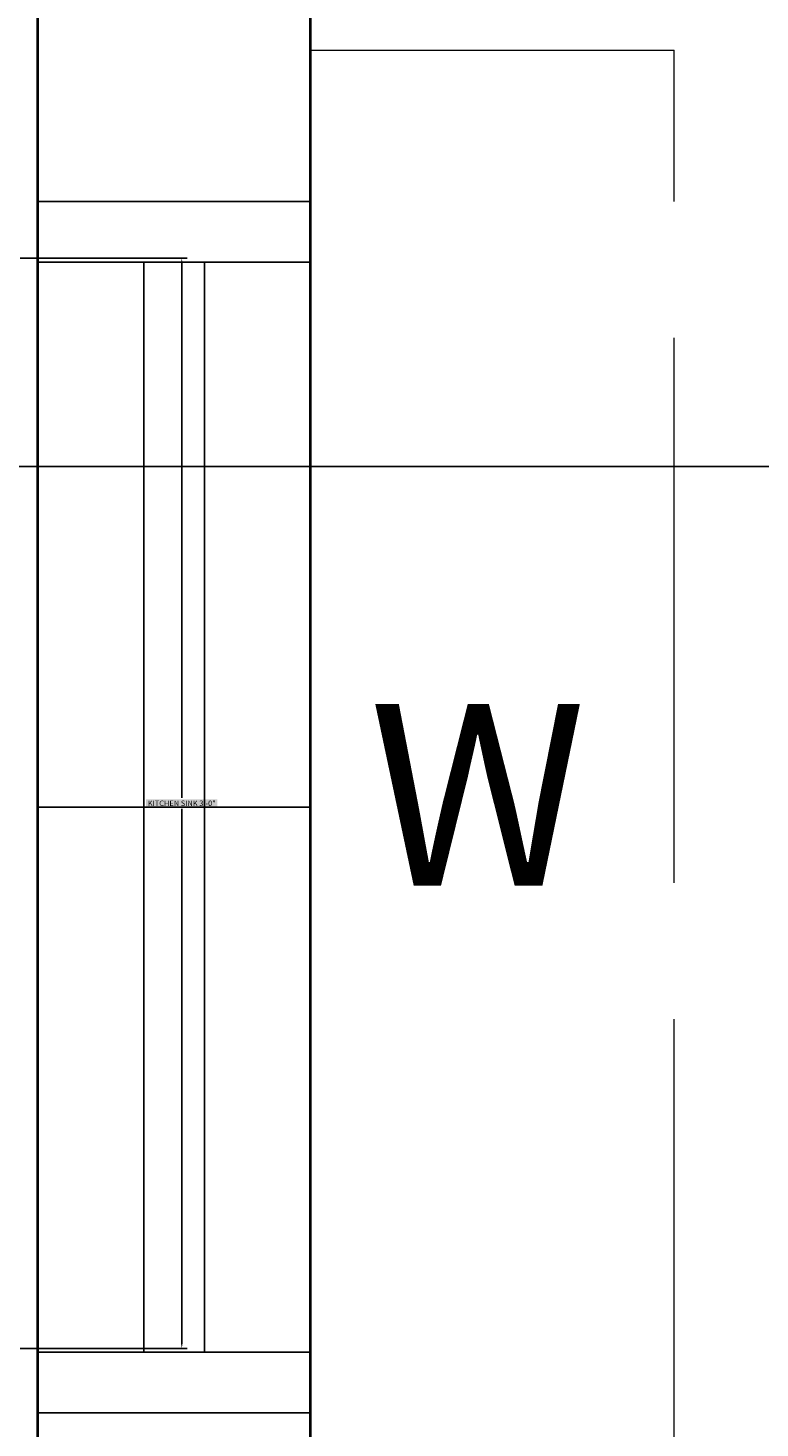
# Model space of a CAD drawing. Units: inches. Extents: x -301 to 715, y -607 to 364.
# Tile 122 of 141: x 124 to 148, y 230 to 276. Entities that reach past the tile are written whole.
import ezdxf

# ---------------------------------------------------------------- set-up
doc = ezdxf.new("R2010")
doc.units = ezdxf.units.IN
doc.header["$MEASUREMENT"] = 0
doc.linetypes.add('ACAD_ISO02W100', pattern=[15, 12, -3])
for name, color, linetype, lineweight in [('A-ANNO-DIMS', 2, 'Continuous', 18), ('A-ANNO-TEXT', 4, 'Continuous', 18), ('A-GLAZ', 2, 'Continuous', 25), ('A-GLAZ-OVHD', 2, 'ACAD_ISO02W100', 18), ('A-WALL', 3, 'Continuous', 40)]:
    doc.layers.add(name, color=color, linetype=linetype, lineweight=lineweight)
doc.styles.get("Standard").update_dxf_attribs({"font": 'arial.ttf'})
doc.dimstyles.get("Standard").update_dxf_attribs({"dimtxt": 0.18, "dimasz": 0.18, "dimexe": 0.18, "dimexo": 0.0625, "dimgap": 0.09, "dimtad": 0, "dimtih": 1, "dimtoh": 1, "dimdec": 1, "dimzin": 0, "dimdsep": 46, "dimlunit": 4, "dimtxsty": 'Standard', "dimcen": 0.09, "dimclrd": 3, "dimclre": 4, "dimclrt": 6, "dimadec": 0, "dimazin": 0, "dimtfac": 1, "dimtdec": 1, "dimtofl": 0, "dimtmove": 0, "dimatfit": 3, "dimfxl": 1, "dimtfill": 2, "dimtfillclr": 51, "dimtolj": 1, "dimtzin": 0, "dimarcsym": 0})

# ---------------------------------------------------------------- blocks, each defined once
blk = doc.blocks.new('WIN-36-PLAN')
for p, q in [((0, 0), (0, 9)), ((2, 0), (2, 9)), ((20, 0), (20, 9)), ((38, 0), (38, 9)), ((40, 0), (40, 9)), ((2, 5.5), (38, 5.5)), ((2, 3.5), (38, 3.5))]:
    blk.add_line(p, q)
blk = doc.blocks.new('WIN-SHADE-50')
at = {"ltscale": 1.5}
for p, q in [((0, 0), (0, 12)), ((50, 12), (0, 12)), ((5, 0), (0, 0)), ((45, 0), (50, 0))]:
    blk.add_line(p, q, dxfattribs=at)
blk = doc.blocks.new('*D142')
at = {"layer": 'A-ANNO-DIMS', "color": 4, "lineweight": -2, "transparency": 16777216}
for p, q in [((123.308, 268.311), (128.826, 268.311)), ((123.308, 232.311), (128.826, 232.311))]:
    blk.add_line(p, q, dxfattribs=at)
at = {"layer": 'A-ANNO-DIMS', "color": 3, "lineweight": -2, "transparency": 16777216}
for p, q in [((128.646, 268.131), (128.646, 250.494)), ((128.646, 232.491), (128.646, 250.128))]:
    blk.add_line(p, q, dxfattribs=at)
at = {"layer": 'A-ANNO-DIMS', "color": 3, "transparency": 16777216}
for points in [[(128.616, 268.131), (128.676, 268.131), (128.646, 268.311)], [(128.616, 232.491), (128.676, 232.491), (128.646, 232.311)]]:
    blk.add_solid(points, dxfattribs=at)
at = {"layer": 'Defpoints', "color": 0, "transparency": 16777216}
for p in [(123.246, 268.311), (128.646, 268.311), (123.246, 232.311)]:
    blk.add_point(p, dxfattribs=at)
at = {"layer": 'A-ANNO-DIMS', "color": 6, "transparency": 16777216, "insert": (128.646, 250.311), "char_height": 0.18, "attachment_point": 5, "bg_fill": 1, "box_fill_scale": 1.25, "bg_fill_color": 51, "bg_fill_transparency": 0}
blk.add_mtext('\\A1;KITCHEN SINK 3\'-0"', dxfattribs=at)
blk = doc.blocks.new('*D153')
at = {"layer": 'A-ANNO-DIMS', "color": 4, "lineweight": -2, "transparency": 16777216}
for p, q in [((132.959, 310.182), (233.659, 310.182)), ((123.959, 193.182), (233.659, 193.182))]:
    blk.add_line(p, q, dxfattribs=at)
at = {"layer": 'A-ANNO-DIMS', "color": 3, "lineweight": -2, "transparency": 16777216}
for p, q in [((233.479, 310.002), (233.479, 251.864)), ((233.479, 193.362), (233.479, 251.5))]:
    blk.add_line(p, q, dxfattribs=at)
at = {"layer": 'A-ANNO-DIMS', "color": 3, "transparency": 16777216}
for points in [[(233.449, 310.002), (233.509, 310.002), (233.479, 310.182)], [(233.449, 193.362), (233.509, 193.362), (233.479, 193.182)]]:
    blk.add_solid(points, dxfattribs=at)
at = {"layer": 'Defpoints', "color": 0, "transparency": 16777216}
for p in [(132.897, 310.182), (123.897, 193.182), (233.479, 193.182)]:
    blk.add_point(p, dxfattribs=at)
at = {"layer": 'A-ANNO-DIMS', "color": 6, "transparency": 16777216, "insert": (233.479, 251.682), "char_height": 0.18, "attachment_point": 5, "bg_fill": 1, "box_fill_scale": 1.25, "bg_fill_color": 51, "bg_fill_transparency": 0}
blk.add_mtext('\\A1;9\'-9"', dxfattribs=at)
blk = doc.blocks.new('*D157')
at = {"layer": 'A-ANNO-DIMS', "color": 4, "lineweight": -2, "transparency": 16777216}
for p, q in [((-50.541, 261.432), (233.659, 261.432)), ((-50.541, 221.682), (233.659, 221.682))]:
    blk.add_line(p, q, dxfattribs=at)
at = {"layer": 'A-ANNO-DIMS', "color": 3, "lineweight": -2, "transparency": 16777216}
for p, q in [((233.479, 261.252), (233.479, 241.739)), ((233.479, 221.862), (233.479, 241.375))]:
    blk.add_line(p, q, dxfattribs=at)
at = {"layer": 'A-ANNO-DIMS', "color": 3, "transparency": 16777216}
for points in [[(233.449, 261.252), (233.509, 261.252), (233.479, 261.432)], [(233.449, 221.862), (233.509, 221.862), (233.479, 221.682)]]:
    blk.add_solid(points, dxfattribs=at)
at = {"layer": 'Defpoints', "color": 0, "transparency": 16777216}
for p in [(-50.603, 261.432), (233.479, 261.432), (-50.603, 221.682)]:
    blk.add_point(p, dxfattribs=at)
at = {"layer": 'A-ANNO-DIMS', "color": 6, "transparency": 16777216, "insert": (233.479, 241.557), "char_height": 0.18, "attachment_point": 5, "bg_fill": 1, "box_fill_scale": 1.25, "bg_fill_color": 51, "bg_fill_transparency": 0}
blk.add_mtext('\\A1;3\'-4"', dxfattribs=at)

msp = doc.modelspace()

# ---------------------------------------------------------------- linework, layer by layer
at = {"layer": 'A-WALL'}
for p, q in [((132.897, 199.182), (132.897, 310.182)), ((123.897, 199.182), (123.897, 301.182))]:
    msp.add_line(p, q, dxfattribs=at)

# ---------------------------------------------------------------- block references
at = {"layer": 'A-GLAZ', "rotation": 90.00000000000026}
msp.add_blockref('WIN-36-PLAN', (132.897, 230.183), dxfattribs=at)
at = {"layer": 'A-GLAZ-OVHD', "rotation": 270.0000000000002}
msp.add_blockref('WIN-SHADE-50', (132.896, 275.182), dxfattribs=at)

# ---------------------------------------------------------------- texts
at = {"layer": 'A-ANNO-TEXT'}
msp.add_text('W', height=6, dxfattribs=at).set_placement((134.82, 247.591))

# ---------------------------------------------------------------- dimensions: what is measured, and where the dimension line sits
at = {"layer": 'A-ANNO-DIMS'}
for base, p1, p2, picture, middle in [((233.479, 193.182), (132.897, 310.182), (123.897, 193.182), '*D153', (233.479, 251.682)), ((233.479242, 261.43233), (-50.603288, 221.68233), (-50.603288, 261.43233), '*D157', (233.479242, 241.55733))]:
    dim = msp.add_linear_dim(base=base, p1=p1, p2=p2, angle=90, dimstyle='Standard', override={"dimdec": 1, "dimlfac": 1, "dimrnd": 0, "dimzin": 1, "dimdsep": 46, "dimlunit": 4, "dimfrac": 2}, dxfattribs=at)
    dim.commit()
    dim.dimension.update_dxf_attribs({"geometry": picture, "text_midpoint": middle})
dim = msp.add_linear_dim(base=(128.646, 268.311), p1=(123.246, 232.311), p2=(123.246, 268.311), angle=90, text='KITCHEN SINK <>', dimstyle='Standard', override={"dimdec": 1, "dimlfac": 1, "dimrnd": 0, "dimzin": 1, "dimdsep": 46, "dimlunit": 4, "dimfrac": 2}, dxfattribs=at)
dim.commit()
dim.dimension.update_dxf_attribs({"geometry": '*D142', "text_midpoint": (128.646, 250.311)})

doc.saveas('drawing.dxf')
